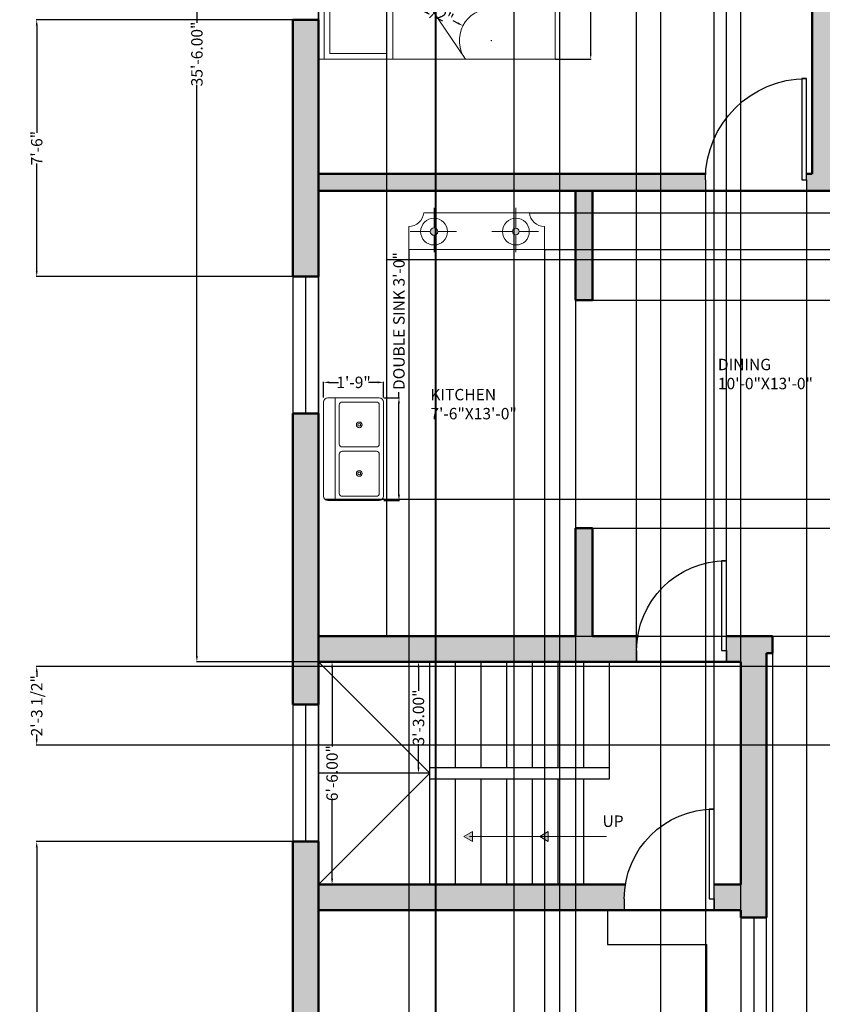
# Model space of a CAD drawing. Units: inches. Extents: x 2430 to 2930, y 1715 to 2575.
# Tile 2 of 4: x 2430 to 2711, y 1933 to 2278. Entities that reach past the tile are written whole.
import ezdxf

# ---------------------------------------------------------------- set-up
doc = ezdxf.new("R2010")
doc.units = ezdxf.units.IN
for name, color, linetype, lineweight in [('A-ANNO-DIMS', 2, 'Continuous', 18), ('A-ANNO-SYMB', 130, 'Continuous', 18), ('A-ANNO-TEXT', 130, 'Continuous', 18), ('A-AREA-IDEN', 130, 'Continuous', 18), ('A-EQPM', 200, 'Continuous', 18), ('A-FLOR', 7, 'Continuous', 25), ('A-FLOR-CASE', 7, 'Continuous', 25), ('A-FLOR-FIXT', 200, 'Continuous', 18), ('A-FLOR-STRS', 7, 'Continuous', 25), ('A-FURN', 200, 'Continuous', 18), ('A-WALL', 7, 'Continuous', 50), ('A-WALL-PATT', 251, 'Continuous', 13), ('DOOR', 224, 'Continuous', 25), ('win', 170, 'Continuous', 25)]:
    doc.layers.add(name, color=color, linetype=linetype, lineweight=lineweight)
doc.styles.get("Standard").update_dxf_attribs({"font": 'arial.ttf', "height": 4})
doc.dimstyles.get("Standard").update_dxf_attribs({"dimtxt": 4, "dimasz": 2, "dimexe": 0.18, "dimexo": 0.0625, "dimgap": 0.09, "dimtad": 0, "dimzin": 0, "dimdsep": 46, "dimlunit": 3, "dimtxsty": 'Standard', "dimcen": 0.09, "dimadec": 0, "dimazin": 0, "dimtfac": 1, "dimtofl": 0, "dimtmove": 0, "dimatfit": 3, "dimfxl": 1, "dimtolj": 1, "dimtzin": 0, "dimarcsym": 0})

# ---------------------------------------------------------------- blocks, each defined once
blk = doc.blocks.new('*D1')
at = {"layer": 'A-ANNO-DIMS', "color": 0, "lineweight": -2, "transparency": 16777216}
for p, q in [((2573.56, 2053.45), (2569.48, 2053.45)), ((2569.66, 2051.45), (2569.66, 2043.24)), ((2569.66, 2016.45), (2569.66, 2024.66)), ((2573.56, 2014.45), (2569.48, 2014.45))]:
    blk.add_line(p, q, dxfattribs=at)
at = {"layer": 'A-ANNO-DIMS', "color": 0, "transparency": 16777216}
for points in [[(2569.32, 2051.45), (2569.99, 2051.45), (2569.66, 2053.45)], [(2569.32, 2016.45), (2569.99, 2016.45), (2569.66, 2014.45)]]:
    blk.add_solid(points, dxfattribs=at)
at = {"layer": 'Defpoints', "color": 0, "transparency": 16777216}
for p in [(2569.66, 2053.45), (2573.62, 2053.45), (2573.62, 2014.45)]:
    blk.add_point(p, dxfattribs=at)
at = {"layer": 'A-ANNO-DIMS', "color": 0, "transparency": 16777216, "insert": (2569.66, 2033.95), "char_height": 4, "attachment_point": 5, "rotation": 90}
blk.add_mtext('\\A1;3\'-3.00"', dxfattribs=at)
blk = doc.blocks.new('*D2')
at = {"layer": 'A-ANNO-DIMS', "color": 0, "lineweight": -2, "transparency": 16777216}
for p, q in [((2534.68, 2053.45), (2539.57, 2053.45)), ((2539.39, 2051.45), (2539.39, 2023.75)), ((2539.39, 1977.45), (2539.39, 2005.15)), ((2534.68, 1975.45), (2539.57, 1975.45))]:
    blk.add_line(p, q, dxfattribs=at)
at = {"layer": 'A-ANNO-DIMS', "color": 0, "transparency": 16777216}
for points in [[(2539.06, 2051.45), (2539.73, 2051.45), (2539.39, 2053.45)], [(2539.06, 1977.45), (2539.73, 1977.45), (2539.39, 1975.45)]]:
    blk.add_solid(points, dxfattribs=at)
at = {"layer": 'Defpoints', "color": 0, "transparency": 16777216}
for p in [(2534.62, 2053.45), (2539.39, 2053.45), (2534.62, 1975.45)]:
    blk.add_point(p, dxfattribs=at)
at = {"layer": 'A-ANNO-DIMS', "color": 0, "transparency": 16777216, "insert": (2539.39, 2014.45), "char_height": 4, "attachment_point": 5, "rotation": 90}
blk.add_mtext('\\A1;6\'-6.00"', dxfattribs=at)
blk = doc.blocks.new('*U5')
for p, q in [((0, 0), (0, -100)), ((800, 0), (800, -100))]:
    blk.add_line(p, q)
blk.add_lwpolyline([(0, 0), (0, 800), (43.75, 800), (43.75, 0)], close=True)
blk.add_arc((0, 0), 800, 0, 90)
blk = doc.blocks.new('*U7')
for p, q in [((0, 0), (0, -100)), ((900, 0), (900, -100))]:
    blk.add_line(p, q)
blk.add_lwpolyline([(0, 0), (0, 900), (43.75, 900), (43.75, 0)], close=True)
blk.add_arc((0, 0), 900, 0, 90)
blk = doc.blocks.new('NEW BED')
for p, q in [((-75.7, 82.92), (0, 82.92)), ((-75.7, 0), (-75.7, 82.92)), ((0, 82.92), (0, 0)), ((-75.7, 80.92), (0, 80.92)), ((-73.7, 78.92), (-39.85, 78.92)), ((-73.7, 58.92), (-73.7, 78.92)), ((-39.85, 58.92), (-39.85, 78.92)), ((-35.85, 78.92), (-2, 78.92)), ((-35.85, 58.92), (-35.85, 78.92)), ((-2, 78.92), (-2, 58.92)), ((-73.7, 58.92), (-39.85, 58.92)), ((-35.85, 58.92), (-2, 58.92)), ((-75.7, 56.92), (0, 56.92)), ((-37.85, 56.92), (-75.7, 31.45)), ((-37.85, 56.92), (-57.85, 22.27)), ((-37.85, 56.92), (0, 31.45)), ((-37.85, 56.92), (-17.84, 22.27)), ((0, 0), (-75.7, 0))]:
    blk.add_line(p, q)
for centre, start, end in [((-69.14, 22.27), 0, 125.5497), ((-6.56, 22.27), 54.4503, 180)]:
    blk.add_arc(centre, 11.28, start, end)
blk = doc.blocks.new('*D13')
at = {"layer": 'A-ANNO-DIMS', "color": 0, "lineweight": -2, "transparency": 16777216}
for p, q in [((2525.56, 2479.45), (2491.85, 2479.45)), ((2492.03, 2477.45), (2492.03, 2277.3)), ((2492.03, 2055.45), (2492.03, 2255.61)), ((2534.56, 2053.45), (2491.85, 2053.45))]:
    blk.add_line(p, q, dxfattribs=at)
at = {"layer": 'A-ANNO-DIMS', "color": 0, "transparency": 16777216}
for points in [[(2491.69, 2477.45), (2492.36, 2477.45), (2492.03, 2479.45)], [(2491.69, 2055.45), (2492.36, 2055.45), (2492.03, 2053.45)]]:
    blk.add_solid(points, dxfattribs=at)
at = {"layer": 'Defpoints', "color": 0, "transparency": 16777216}
for p in [(2525.62, 2479.45), (2492.03, 2053.45), (2534.62, 2053.45)]:
    blk.add_point(p, dxfattribs=at)
at = {"layer": 'A-ANNO-DIMS', "color": 0, "transparency": 16777216, "insert": (2492.03, 2266.45), "char_height": 4, "attachment_point": 5, "rotation": 90}
blk.add_mtext('\\A1;35\'-6.00"', dxfattribs=at)
blk = doc.blocks.new('Sink-double - 36 in top')
for p, q in [((-18, -4), (18, -4)), ((-0.75, -18.5), (-0.75, -6.5)), ((0.75, -6.5), (0.75, -18.5))]:
    blk.add_line(p, q)
for points in [[(-16.5, 0), (16.5, 0)], [(-18, -19.5), (-18, -1.5)], [(18, -1.5), (18, -19.5)], [(-16.5, -18.5), (-16.5, -6.5)], [(-15.5, -5.5), (-1.75, -5.5)], [(1.75, -5.5), (15.5, -5.5)], [(16.5, -6.5), (16.5, -18.5)], [(-1.75, -19.5), (-15.5, -19.5)], [(15.5, -19.5), (1.75, -19.5)], [(16.5, -21), (-16.5, -21)]]:
    blk.add_lwpolyline(points)
for centre, radius in [((-8.5, -12.5), 1), ((-8.5, -12.5), 0.5), ((8.5, -12.5), 1), ((8.5, -12.5), 0.5)]:
    blk.add_circle(centre, radius)
for centre, radius, start, end in [((-16.5, -1.5), 1.5, 90, 180), ((16.5, -1.5), 1.5, 0, 90), ((-15.5, -6.5), 1, 90, 180), ((-1.75, -6.5), 1, 0, 90), ((1.75, -6.5), 1, 90, 180), ((15.5, -6.5), 1, 0, 90), ((-16.5, -19.5), 1.5, 180, 270), ((-15.5, -18.5), 1, 180, 270), ((-1.75, -18.5), 1, 270, 0), ((1.75, -18.5), 1, 180, 270), ((15.5, -18.5), 1, 270, 0), ((16.5, -19.5), 1.5, 270, 0)]:
    blk.add_arc(centre, radius, start, end)
blk = doc.blocks.new('WIN-48IN')
blk.add_line((0, 4.5), (48, 4.5))
blk.add_lwpolyline([(0, 9), (48, 9), (48, 0), (0, 0)], close=True)
blk = doc.blocks.new('*D22')
at = {"layer": 'A-ANNO-DIMS', "color": 0, "lineweight": -2, "transparency": 16777216}
for p, q in [((2617.61, 2340.3), (2630.16, 2340.3)), ((2629.98, 2338.3), (2629.98, 2319.41)), ((2629.98, 2266.6), (2629.98, 2285.5)), ((2617.61, 2264.6), (2630.16, 2264.6))]:
    blk.add_line(p, q, dxfattribs=at)
at = {"layer": 'A-ANNO-DIMS', "color": 0, "transparency": 16777216}
for points in [[(2629.65, 2338.3), (2630.31, 2338.3), (2629.98, 2340.3)], [(2629.65, 2266.6), (2630.31, 2266.6), (2629.98, 2264.6)]]:
    blk.add_solid(points, dxfattribs=at)
at = {"layer": 'Defpoints', "color": 0, "transparency": 16777216}
for p in [(2617.54, 2340.3), (2629.98, 2340.3), (2617.54, 2264.6)]:
    blk.add_point(p, dxfattribs=at)
at = {"layer": 'A-ANNO-DIMS', "color": 0, "transparency": 16777216, "insert": (2629.98, 2302.45), "char_height": 4, "attachment_point": 5, "rotation": 90}
blk.add_mtext('\\A1;6\'-3 1/2" TYP.', dxfattribs=at)
blk = doc.blocks.new('*D23')
at = {"layer": 'A-ANNO-DIMS', "color": 0, "lineweight": -2, "transparency": 16777216}
for p, q in [((2557.48, 2145.98), (2562.99, 2145.98)), ((2562.81, 2145.98), (2562.81, 2147.98)), ((2562.81, 2111.98), (2562.81, 2143.98)), ((2557.48, 2109.98), (2562.99, 2109.98))]:
    blk.add_line(p, q, dxfattribs=at)
at = {"layer": 'A-ANNO-DIMS', "color": 0, "transparency": 16777216}
for points in [[(2562.48, 2143.98), (2563.15, 2143.98), (2562.81, 2145.98)], [(2562.48, 2111.98), (2563.15, 2111.98), (2562.81, 2109.98)]]:
    blk.add_solid(points, dxfattribs=at)
at = {"layer": 'Defpoints', "color": 0, "transparency": 16777216}
for p in [(2557.41, 2145.98), (2562.81, 2145.98), (2557.41, 2109.98)]:
    blk.add_point(p, dxfattribs=at)
at = {"layer": 'A-ANNO-DIMS', "color": 0, "transparency": 16777216, "insert": (2562.81, 2172.85), "char_height": 4, "attachment_point": 5, "rotation": 90}
blk.add_mtext('\\A1;DOUBLE SINK 3\'-0"', dxfattribs=at)
blk = doc.blocks.new('*D24')
at = {"layer": 'A-ANNO-DIMS', "color": 0, "lineweight": -2, "transparency": 16777216}
for p, q in [((2536.41, 2146.05), (2536.41, 2151.56)), ((2538.41, 2151.38), (2541.69, 2151.38)), ((2555.41, 2151.38), (2552.13, 2151.38)), ((2557.41, 2146.05), (2557.41, 2151.56))]:
    blk.add_line(p, q, dxfattribs=at)
at = {"layer": 'A-ANNO-DIMS', "color": 0, "transparency": 16777216}
for points in [[(2538.41, 2151.72), (2538.41, 2151.05), (2536.41, 2151.38)], [(2555.41, 2151.72), (2555.41, 2151.05), (2557.41, 2151.38)]]:
    blk.add_solid(points, dxfattribs=at)
at = {"layer": 'Defpoints', "color": 0, "transparency": 16777216}
for p in [(2536.41, 2151.38), (2536.41, 2145.98), (2557.41, 2145.98)]:
    blk.add_point(p, dxfattribs=at)
at = {"layer": 'A-ANNO-DIMS', "color": 0, "transparency": 16777216, "insert": (2546.91, 2151.38), "char_height": 4, "attachment_point": 5}
blk.add_mtext('\\A1;1\'-9"', dxfattribs=at)
blk = doc.blocks.new('*D26')
at = {"layer": 'A-ANNO-DIMS', "color": 0, "lineweight": -2, "transparency": 16777216}
for p, q in [((2786.56, 2051.85), (2435.74, 2051.85)), ((2435.92, 2049.85), (2435.92, 2048.17)), ((2435.92, 2026.29), (2435.92, 2027.97)), ((2786.56, 2024.29), (2435.74, 2024.29))]:
    blk.add_line(p, q, dxfattribs=at)
at = {"layer": 'A-ANNO-DIMS', "color": 0, "transparency": 16777216}
for points in [[(2435.59, 2049.85), (2436.25, 2049.85), (2435.92, 2051.85)], [(2435.59, 2026.29), (2436.25, 2026.29), (2435.92, 2024.29)]]:
    blk.add_solid(points, dxfattribs=at)
at = {"layer": 'Defpoints', "color": 0, "transparency": 16777216}
for p in [(2435.92, 2051.85), (2786.62, 2051.85), (2786.62, 2024.29)]:
    blk.add_point(p, dxfattribs=at)
at = {"layer": 'A-ANNO-DIMS', "color": 0, "transparency": 16777216, "insert": (2435.92, 2038.07), "char_height": 4, "attachment_point": 5, "rotation": 90}
blk.add_mtext('\\A1;2\'-3 1/2"', dxfattribs=at)
blk = doc.blocks.new('*D30')
at = {"layer": 'A-ANNO-DIMS', "color": 0, "lineweight": -2, "transparency": 16777216}
for p, q in [((2534.62, 2470.39), (2534.62, 1720.57)), ((2575.68, 2470.39), (2575.68, 1720.57)), ((2536.62, 1720.75), (2549.75, 1720.75)), ((2573.68, 1720.75), (2560.56, 1720.75))]:
    blk.add_line(p, q, dxfattribs=at)
at = {"layer": 'A-ANNO-DIMS', "color": 0, "transparency": 16777216}
for points in [[(2536.62, 1721.09), (2536.62, 1720.42), (2534.62, 1720.75)], [(2573.68, 1721.09), (2573.68, 1720.42), (2575.68, 1720.75)]]:
    blk.add_solid(points, dxfattribs=at)
at = {"layer": 'Defpoints', "color": 0, "transparency": 16777216}
for p in [(2534.62, 2470.45), (2575.68, 2470.45), (2575.68, 1720.75)]:
    blk.add_point(p, dxfattribs=at)
at = {"layer": 'A-ANNO-DIMS', "color": 0, "transparency": 16777216, "insert": (2555.15, 1720.75), "char_height": 4, "attachment_point": 5}
blk.add_mtext('\\A1;3\'-5"', dxfattribs=at)
blk = doc.blocks.new('*D33')
at = {"layer": 'A-ANNO-DIMS', "color": 0, "lineweight": -2, "transparency": 16777216}
for p, q in [((2525.56, 2278.45), (2435.74, 2278.45)), ((2435.92, 2276.45), (2435.92, 2238.84)), ((2435.92, 2190.45), (2435.92, 2228.06)), ((2525.56, 2188.45), (2435.74, 2188.45))]:
    blk.add_line(p, q, dxfattribs=at)
at = {"layer": 'A-ANNO-DIMS', "color": 0, "transparency": 16777216}
for points in [[(2435.59, 2276.45), (2436.25, 2276.45), (2435.92, 2278.45)], [(2435.59, 2190.45), (2436.25, 2190.45), (2435.92, 2188.45)]]:
    blk.add_solid(points, dxfattribs=at)
at = {"layer": 'Defpoints', "color": 0, "transparency": 16777216}
for p in [(2525.62, 2278.45), (2435.92, 2188.45), (2525.62, 2188.45)]:
    blk.add_point(p, dxfattribs=at)
at = {"layer": 'A-ANNO-DIMS', "color": 0, "transparency": 16777216, "insert": (2435.92, 2233.45), "char_height": 4, "attachment_point": 5, "rotation": 90}
blk.add_mtext('\\A1;7\'-6"', dxfattribs=at)
blk = doc.blocks.new('*D34')
at = {"layer": 'A-ANNO-DIMS', "color": 0, "lineweight": -2, "transparency": 16777216}
for p, q in [((2525.56, 1990.45), (2435.74, 1990.45)), ((2435.92, 1988.45), (2435.92, 1881.72)), ((2435.92, 1761.45), (2435.92, 1868.18)), ((2525.56, 1759.45), (2435.74, 1759.45))]:
    blk.add_line(p, q, dxfattribs=at)
at = {"layer": 'A-ANNO-DIMS', "color": 0, "transparency": 16777216}
for points in [[(2435.59, 1988.45), (2436.25, 1988.45), (2435.92, 1990.45)], [(2435.59, 1761.45), (2436.25, 1761.45), (2435.92, 1759.45)]]:
    blk.add_solid(points, dxfattribs=at)
at = {"layer": 'Defpoints', "color": 0, "transparency": 16777216}
for p in [(2435.92, 1990.45), (2525.62, 1990.45), (2525.62, 1759.45)]:
    blk.add_point(p, dxfattribs=at)
at = {"layer": 'A-ANNO-DIMS', "color": 0, "transparency": 16777216, "insert": (2435.92, 1874.95), "char_height": 4, "attachment_point": 5, "rotation": 90}
blk.add_mtext('\\A1;19\'-3"', dxfattribs=at)
blk = doc.blocks.new('*D40')
at = {"layer": 'A-ANNO-DIMS', "color": 0, "lineweight": -2, "transparency": 16777216}
for p, q in [((2630.68, 2180.15), (2924.5, 2180.15)), ((2924.32, 2178.15), (2924.32, 2145.66)), ((2924.32, 2102.32), (2924.32, 2134.82)), ((2630.68, 2100.32), (2924.5, 2100.32))]:
    blk.add_line(p, q, dxfattribs=at)
at = {"layer": 'A-ANNO-DIMS', "color": 0, "transparency": 16777216}
for points in [[(2923.99, 2178.15), (2924.65, 2178.15), (2924.32, 2180.15)], [(2923.99, 2102.32), (2924.65, 2102.32), (2924.32, 2100.32)]]:
    blk.add_solid(points, dxfattribs=at)
at = {"layer": 'Defpoints', "color": 0, "transparency": 16777216}
for p in [(2630.62, 2180.15), (2924.32, 2180.15), (2630.62, 2100.32)]:
    blk.add_point(p, dxfattribs=at)
at = {"layer": 'A-ANNO-DIMS', "color": 0, "transparency": 16777216, "insert": (2924.32, 2140.24), "char_height": 4, "attachment_point": 5, "rotation": 90}
blk.add_mtext('\\A1;6\'-8"', dxfattribs=at)
blk = doc.blocks.new('*D41')
at = {"layer": 'A-ANNO-DIMS', "color": 0, "lineweight": -2, "transparency": 16777216}
for p, q in [((2693.62, 2062.39), (2693.62, 1720.57)), ((2750.62, 2056.39), (2750.62, 1720.57)), ((2695.62, 1720.75), (2716.63, 1720.75)), ((2748.62, 1720.75), (2727.61, 1720.75))]:
    blk.add_line(p, q, dxfattribs=at)
at = {"layer": 'A-ANNO-DIMS', "color": 0, "transparency": 16777216}
for points in [[(2695.62, 1721.09), (2695.62, 1720.42), (2693.62, 1720.75)], [(2748.62, 1721.09), (2748.62, 1720.42), (2750.62, 1720.75)]]:
    blk.add_solid(points, dxfattribs=at)
at = {"layer": 'Defpoints', "color": 0, "transparency": 16777216}
for p in [(2693.62, 2062.45), (2750.62, 2056.45), (2750.62, 1720.75)]:
    blk.add_point(p, dxfattribs=at)
at = {"layer": 'A-ANNO-DIMS', "color": 0, "transparency": 16777216, "insert": (2722.12, 1720.75), "char_height": 4, "attachment_point": 5}
blk.add_mtext('\\A1;4\'-9"', dxfattribs=at)
blk = doc.blocks.new('*D42')
at = {"layer": 'A-ANNO-DIMS', "color": 0, "lineweight": -2, "transparency": 16777216}
for p, q in [((2646.07, 2053.52), (2646.07, 2569.33)), ((2648.07, 2569.15), (2651.72, 2569.15)), ((2675.57, 2569.15), (2671.92, 2569.15)), ((2677.57, 2053.52), (2677.57, 2569.33))]:
    blk.add_line(p, q, dxfattribs=at)
at = {"layer": 'A-ANNO-DIMS', "color": 0, "transparency": 16777216}
for points in [[(2648.07, 2569.49), (2648.07, 2568.82), (2646.07, 2569.15)], [(2675.57, 2569.49), (2675.57, 2568.82), (2677.57, 2569.15)]]:
    blk.add_solid(points, dxfattribs=at)
at = {"layer": 'Defpoints', "color": 0, "transparency": 16777216}
for p in [(2677.57, 2569.15), (2646.07, 2053.45), (2677.57, 2053.45)]:
    blk.add_point(p, dxfattribs=at)
at = {"layer": 'A-ANNO-DIMS', "color": 0, "transparency": 16777216, "insert": (2661.82, 2569.15), "char_height": 4, "attachment_point": 5}
blk.add_mtext('\\A1;2\'-7 1/2"', dxfattribs=at)
blk = doc.blocks.new('*D43')
at = {"layer": 'A-ANNO-DIMS', "color": 0, "lineweight": -2, "transparency": 16777216}
for p, q in [((2673.24, 1966.52), (2673.24, 2569.33)), ((2675.24, 2569.15), (2680.62, 2569.15)), ((2682.62, 1966.52), (2682.62, 2569.33)), ((2682.62, 2569.15), (2684.62, 2569.15))]:
    blk.add_line(p, q, dxfattribs=at)
at = {"layer": 'A-ANNO-DIMS', "color": 0, "transparency": 16777216}
for points in [[(2675.24, 2569.49), (2675.24, 2568.82), (2673.24, 2569.15)], [(2680.62, 2569.49), (2680.62, 2568.82), (2682.62, 2569.15)]]:
    blk.add_solid(points, dxfattribs=at)
at = {"layer": 'Defpoints', "color": 0, "transparency": 16777216}
for p in [(2682.62, 2569.15), (2673.24, 1966.45), (2682.62, 1966.45)]:
    blk.add_point(p, dxfattribs=at)
at = {"layer": 'A-ANNO-DIMS', "color": 0, "transparency": 16777216, "insert": (2694.69, 2569.15), "char_height": 4, "attachment_point": 5}
blk.add_mtext('\\A1;0\'-9 1/2"', dxfattribs=at)
blk = doc.blocks.new('*D44')
at = {"layer": 'A-ANNO-DIMS', "color": 0, "lineweight": -2, "transparency": 16777216}
for p, q in [((2670.19, 2218.39), (2670.19, 1720.57)), ((2705.62, 2218.39), (2705.62, 1720.57)), ((2672.19, 1720.75), (2676.25, 1720.75)), ((2703.62, 1720.75), (2699.56, 1720.75))]:
    blk.add_line(p, q, dxfattribs=at)
at = {"layer": 'A-ANNO-DIMS', "color": 0, "transparency": 16777216}
for points in [[(2672.19, 1721.09), (2672.19, 1720.42), (2670.19, 1720.75)], [(2703.62, 1721.09), (2703.62, 1720.42), (2705.62, 1720.75)]]:
    blk.add_solid(points, dxfattribs=at)
at = {"layer": 'Defpoints', "color": 0, "transparency": 16777216}
for p in [(2670.19, 2218.45), (2705.62, 2218.45), (2670.19, 1720.75)]:
    blk.add_point(p, dxfattribs=at)
at = {"layer": 'A-ANNO-DIMS', "color": 0, "transparency": 16777216, "insert": (2687.9, 1720.75), "char_height": 4, "attachment_point": 5}
blk.add_mtext('\\A1;2\'-11 1/2"', dxfattribs=at)
blk = doc.blocks.new('*D45')
at = {"layer": 'A-ANNO-DIMS', "color": 0, "lineweight": -2, "transparency": 16777216}
for p, q in [((2619.01, 2380.39), (2619.01, 1720.57)), ((2654.44, 2380.39), (2654.44, 1720.57)), ((2621.01, 1720.75), (2625.07, 1720.75)), ((2652.44, 1720.75), (2648.38, 1720.75))]:
    blk.add_line(p, q, dxfattribs=at)
at = {"layer": 'A-ANNO-DIMS', "color": 0, "transparency": 16777216}
for points in [[(2621.01, 1721.09), (2621.01, 1720.42), (2619.01, 1720.75)], [(2652.44, 1721.09), (2652.44, 1720.42), (2654.44, 1720.75)]]:
    blk.add_solid(points, dxfattribs=at)
at = {"layer": 'Defpoints', "color": 0, "transparency": 16777216}
for p in [(2619.01, 2380.45), (2654.44, 2380.45), (2654.44, 1720.75)]:
    blk.add_point(p, dxfattribs=at)
at = {"layer": 'A-ANNO-DIMS', "color": 0, "transparency": 16777216, "insert": (2636.72, 1720.75), "char_height": 4, "attachment_point": 5}
blk.add_mtext('\\A1;2\'-11 1/2"', dxfattribs=at)
blk = doc.blocks.new('*D46')
at = {"layer": 'A-ANNO-DIMS', "color": 0, "lineweight": -2, "transparency": 16777216}
for p, q in [((2575.5, 2380.39), (2575.5, 1720.57)), ((2603.06, 2380.39), (2603.06, 1720.57)), ((2577.5, 1720.75), (2579.18, 1720.75)), ((2601.06, 1720.75), (2599.38, 1720.75))]:
    blk.add_line(p, q, dxfattribs=at)
at = {"layer": 'A-ANNO-DIMS', "color": 0, "transparency": 16777216}
for points in [[(2577.5, 1721.09), (2577.5, 1720.42), (2575.5, 1720.75)], [(2601.06, 1721.09), (2601.06, 1720.42), (2603.06, 1720.75)]]:
    blk.add_solid(points, dxfattribs=at)
at = {"layer": 'Defpoints', "color": 0, "transparency": 16777216}
for p in [(2575.5, 2380.45), (2603.06, 2380.45), (2603.06, 1720.75)]:
    blk.add_point(p, dxfattribs=at)
at = {"layer": 'A-ANNO-DIMS', "color": 0, "transparency": 16777216, "insert": (2589.28, 1720.75), "char_height": 4, "attachment_point": 5}
blk.add_mtext('\\A1;2\'-3 1/2"', dxfattribs=at)
blk = doc.blocks.new('*D49')
at = {"layer": 'A-ANNO-DIMS', "color": 0, "lineweight": -2, "transparency": 16777216}
for p, q in [((2534.62, 2062.52), (2534.62, 2569.33)), ((2536.62, 2569.15), (2541.18, 2569.15)), ((2556.62, 2569.15), (2552.06, 2569.15)), ((2558.62, 2062.52), (2558.62, 2569.33))]:
    blk.add_line(p, q, dxfattribs=at)
at = {"layer": 'A-ANNO-DIMS', "color": 0, "transparency": 16777216}
for points in [[(2536.62, 2569.49), (2536.62, 2568.82), (2534.62, 2569.15)], [(2556.62, 2569.49), (2556.62, 2568.82), (2558.62, 2569.15)]]:
    blk.add_solid(points, dxfattribs=at)
at = {"layer": 'Defpoints', "color": 0, "transparency": 16777216}
for p in [(2558.62, 2569.15), (2534.62, 2062.45), (2558.62, 2062.45)]:
    blk.add_point(p, dxfattribs=at)
at = {"layer": 'A-ANNO-DIMS', "color": 0, "transparency": 16777216, "insert": (2546.62, 2569.15), "char_height": 4, "attachment_point": 5}
blk.add_mtext('\\A1;2\'-0"', dxfattribs=at)
blk = doc.blocks.new('*D50')
at = {"layer": 'A-ANNO-DIMS', "color": 0, "lineweight": -2, "transparency": 16777216}
for p, q in [((2536.91, 2110.42), (2924.5, 2110.42)), ((2924.32, 2108.42), (2924.32, 2091.92)), ((2924.32, 2064.45), (2924.32, 2080.95)), ((2534.68, 2062.45), (2924.5, 2062.45))]:
    blk.add_line(p, q, dxfattribs=at)
at = {"layer": 'A-ANNO-DIMS', "color": 0, "transparency": 16777216}
for points in [[(2923.99, 2108.42), (2924.65, 2108.42), (2924.32, 2110.42)], [(2923.99, 2064.45), (2924.65, 2064.45), (2924.32, 2062.45)]]:
    blk.add_solid(points, dxfattribs=at)
at = {"layer": 'Defpoints', "color": 0, "transparency": 16777216}
for p in [(2536.85, 2110.42), (2534.62, 2062.45), (2924.32, 2062.45)]:
    blk.add_point(p, dxfattribs=at)
at = {"layer": 'A-ANNO-DIMS', "color": 0, "transparency": 16777216, "insert": (2924.32, 2086.44), "char_height": 4, "attachment_point": 5, "rotation": 90}
blk.add_mtext('\\A1;4\'-0"', dxfattribs=at)
blk = doc.blocks.new('*D51')
at = {"layer": 'A-ANNO-DIMS', "color": 0, "lineweight": -2, "transparency": 16777216}
for p, q in [((2566.24, 2197.83), (2566.24, 1720.57)), ((2613.75, 2197.83), (2613.75, 1720.57)), ((2568.24, 1720.75), (2578.38, 1720.75)), ((2611.75, 1720.75), (2601.62, 1720.75))]:
    blk.add_line(p, q, dxfattribs=at)
at = {"layer": 'A-ANNO-DIMS', "color": 0, "transparency": 16777216}
for points in [[(2568.24, 1721.09), (2568.24, 1720.42), (2566.24, 1720.75)], [(2611.75, 1721.09), (2611.75, 1720.42), (2613.75, 1720.75)]]:
    blk.add_solid(points, dxfattribs=at)
at = {"layer": 'Defpoints', "color": 0, "transparency": 16777216}
for p in [(2566.24, 2197.89), (2613.75, 2197.89), (2613.75, 1720.75)]:
    blk.add_point(p, dxfattribs=at)
at = {"layer": 'A-ANNO-DIMS', "color": 0, "transparency": 16777216, "insert": (2590, 1720.75), "char_height": 4, "attachment_point": 5}
blk.add_mtext('\\A1;3\'-11 1/2"', dxfattribs=at)
blk = doc.blocks.new('*D52')
at = {"layer": 'A-ANNO-DIMS', "color": 0, "lineweight": -2, "transparency": 16777216}
for p, q in [((2924.32, 2212.78), (2924.32, 2214.78)), ((2608.57, 2210.78), (2924.5, 2210.78)), ((2613.81, 2197.89), (2924.5, 2197.89)), ((2924.32, 2195.89), (2924.32, 2193.89))]:
    blk.add_line(p, q, dxfattribs=at)
at = {"layer": 'A-ANNO-DIMS', "color": 0, "transparency": 16777216}
for points in [[(2923.99, 2212.78), (2924.65, 2212.78), (2924.32, 2210.78)], [(2923.99, 2195.89), (2924.65, 2195.89), (2924.32, 2197.89)]]:
    blk.add_solid(points, dxfattribs=at)
at = {"layer": 'Defpoints', "color": 0, "transparency": 16777216}
for p in [(2608.51, 2210.78), (2924.32, 2210.78), (2613.75, 2197.89)]:
    blk.add_point(p, dxfattribs=at)
at = {"layer": 'A-ANNO-DIMS', "color": 0, "transparency": 16777216, "insert": (2924.32, 2204.34), "char_height": 4, "attachment_point": 5, "rotation": 90}
blk.add_mtext('\\A1;1\'-1"', dxfattribs=at)
blk = doc.blocks.new('*D53')
at = {"layer": 'A-ANNO-DIMS', "color": 0, "lineweight": -2, "transparency": 16777216}
for p, q in [((2613.75, 2197.83), (2613.75, 1720.57)), ((2624.62, 2194.39), (2624.62, 1720.57)), ((2615.75, 1720.75), (2622.62, 1720.75)), ((2624.62, 1720.75), (2626.62, 1720.75))]:
    blk.add_line(p, q, dxfattribs=at)
at = {"layer": 'A-ANNO-DIMS', "color": 0, "transparency": 16777216}
for points in [[(2615.75, 1721.09), (2615.75, 1720.42), (2613.75, 1720.75)], [(2622.62, 1721.09), (2622.62, 1720.42), (2624.62, 1720.75)]]:
    blk.add_solid(points, dxfattribs=at)
at = {"layer": 'Defpoints', "color": 0, "transparency": 16777216}
for p in [(2613.75, 2197.89), (2624.62, 2194.45), (2624.62, 1720.75)]:
    blk.add_point(p, dxfattribs=at)
at = {"layer": 'A-ANNO-DIMS', "color": 0, "transparency": 16777216, "insert": (2633.58, 1720.75), "char_height": 4, "attachment_point": 5}
blk.add_mtext('\\A1;0\'-11"', dxfattribs=at)
blk = doc.blocks.new('*D54')
at = {"layer": 'A-ANNO-DIMS', "color": 0, "lineweight": -2, "transparency": 16777216}
for p, q in [((2624.68, 2218.45), (2924.5, 2218.45)), ((2924.32, 2216.45), (2924.32, 2211.89)), ((2924.32, 2196.45), (2924.32, 2201.01)), ((2624.68, 2194.45), (2924.5, 2194.45))]:
    blk.add_line(p, q, dxfattribs=at)
at = {"layer": 'A-ANNO-DIMS', "color": 0, "transparency": 16777216}
for points in [[(2923.99, 2216.45), (2924.65, 2216.45), (2924.32, 2218.45)], [(2923.99, 2196.45), (2924.65, 2196.45), (2924.32, 2194.45)]]:
    blk.add_solid(points, dxfattribs=at)
at = {"layer": 'Defpoints', "color": 0, "transparency": 16777216}
for p in [(2624.62, 2218.45), (2924.32, 2218.45), (2624.62, 2194.45)]:
    blk.add_point(p, dxfattribs=at)
at = {"layer": 'A-ANNO-DIMS', "color": 0, "transparency": 16777216, "insert": (2924.32, 2206.45), "char_height": 4, "attachment_point": 5, "rotation": 90}
blk.add_mtext('\\A1;2\'-0"', dxfattribs=at)
blk = doc.blocks.new('*D55')
at = {"layer": 'A-ANNO-DIMS', "color": 0, "lineweight": -2, "transparency": 16777216}
for p, q in [((2581.68, 2278.16), (2583.46, 2277.24)), ((2595.18, 2271.16), (2595.36, 2271.16)), ((2595.27, 2271.07), (2595.27, 2271.25))]:
    blk.add_line(p, q, dxfattribs=at)
at = {"layer": 'A-ANNO-DIMS', "color": 0, "transparency": 16777216}
blk.add_solid([(2583.61, 2277.54), (2583.31, 2276.94), (2585.24, 2276.33)], dxfattribs=at)
at = {"layer": 'Defpoints', "color": 0, "transparency": 16777216}
for p in [(2585.24, 2276.33), (2595.27, 2271.16)]:
    blk.add_point(p, dxfattribs=at)
at = {"layer": 'A-ANNO-DIMS', "color": 0, "transparency": 16777216, "insert": (2565.79, 2286.33), "char_height": 4, "attachment_point": 5, "rotation": 332.7752}
blk.add_mtext('\\A1;2X R0\'-11 1/2"', dxfattribs=at)

msp = doc.modelspace()

# ---------------------------------------------------------------- hatches: boundary and pattern name
at = {"layer": 'A-ANNO-SYMB'}
h = msp.add_hatch(color=256, dxfattribs=at)
h.dxf.hatch_style = 1
h.paths.add_polyline_path([(2588.532, 1993.979), (2585.551, 1992.258), (2588.532, 1990.536)])
h.paths.add_polyline_path([(2612.155, 1992.258), (2615.136, 1992.258), (2615.136, 1993.979)])
h.paths.add_polyline_path([(2612.155, 1992.258), (2615.136, 1990.536), (2615.136, 1992.258)])
at = {"layer": 'A-EQPM'}
h = msp.add_hatch(color=256, dxfattribs=at)
h.dxf.hatch_style = 1
h.paths.add_polyline_path([(2602.635, 2204.204, 1), (2604.959, 2204.204, 1)])
h.paths.add_polyline_path([(2576.398, 2204.204, 1), (2573.799, 2204.204, 1)])
at = {"layer": 'A-WALL-PATT'}
h = msp.add_hatch(color=256, dxfattribs=at)
h.dxf.hatch_style = 1
h.paths.add_polyline_path([(2714.621, 2380.453), (2707.621, 2380.453), (2707.621, 2224.453), (2705.621, 2224.453), (2705.621, 2222.39), (2705.621, 2218.453), (2715.188, 2218.453), (2715.188, 2222.39), (2715.188, 2224.453), (2714.621, 2224.453)])
h.paths.add_polyline_path([(2756.969, 2384.39, -0.0145648), (2757.029, 2386.453), (2654.378, 2386.453, -0.0145648), (2654.438, 2384.39), (2654.438, 2380.453), (2756.969, 2380.453)])
h = msp.add_hatch(color=256, dxfattribs=at)
h.dxf.hatch_style = 1
h.paths.add_polyline_path([(2885.621, 2116.453), (2876.621, 2116.453), (2876.621, 2044.453), (2885.621, 2044.453)])
h.paths.add_polyline_path([(2876.621, 2062.453), (2756.621, 2062.453), (2756.621, 2065.333), (2754.558, 2065.333), (2750.621, 2065.333), (2750.621, 2062.453), (2750.621, 2056.453), (2876.621, 2056.453)])
h.paths.add_polyline_path([(2885.621, 2278.453), (2876.621, 2278.453), (2876.621, 2164.453), (2885.621, 2164.453)])
h.paths.add_polyline_path([(2876.621, 2224.453), (2750.561, 2224.453, -0.0145648), (2750.621, 2222.39), (2750.621, 2218.453), (2876.621, 2218.453)])
h.paths.add_polyline_path([(2756.621, 2218.453), (2750.621, 2218.453), (2750.621, 2100.766), (2754.558, 2100.766, -0.0145648), (2756.621, 2100.706)])
h.paths.add_polyline_path([(2630.621, 2100.325), (2624.621, 2100.325), (2624.621, 2062.453), (2534.621, 2062.453), (2534.621, 2053.453), (2646.072, 2053.453), (2646.072, 2057.39, -0.0403846), (2646.482, 2062.453), (2630.621, 2062.453)])
h.paths.add_polyline_path([(2534.621, 2140.453), (2525.621, 2140.453), (2525.621, 2038.453), (2534.621, 2038.453)])
h.paths.add_polyline_path([(2670.188, 2222.39, -0.0145648), (2670.248, 2224.453), (2534.621, 2224.453), (2534.621, 2218.453), (2670.188, 2218.453)])
h.paths.add_polyline_path([(2630.621, 2218.453), (2624.621, 2218.453), (2624.621, 2180.154), (2630.621, 2180.154)])
h.paths.add_polyline_path([(2534.621, 2278.453), (2525.621, 2278.453), (2525.621, 2188.453), (2534.621, 2188.453)])
h = msp.add_hatch(color=256, dxfattribs=at)
h.dxf.hatch_style = 1
h.paths.add_polyline_path([(2885.621, 1897.453), (2876.621, 1897.453), (2876.621, 1769.453), (2682.621, 1769.453), (2682.621, 1759.453), (2885.621, 1759.453)])
h.paths.add_polyline_path([(2885.621, 2020.453), (2876.621, 2020.453), (2876.621, 1945.453), (2885.621, 1945.453)])
h.paths.add_polyline_path([(2876.621, 1840.453), (2808.121, 1840.453), (2808.121, 1831.453), (2876.621, 1831.453)], flags=17)
h.paths.add_polyline_path([(2760.121, 1840.453), (2691.621, 1840.453), (2691.621, 1849.896), (2686.558, 1849.896), (2682.621, 1849.896), (2682.621, 1831.453), (2760.121, 1831.453)], flags=17)
h.paths.add_polyline_path([(2691.621, 1915.889), (2682.621, 1915.889), (2682.621, 1889.266), (2686.558, 1889.266, -0.0322505), (2691.621, 1888.939)])
h.paths.add_polyline_path([(2691.621, 2056.453), (2693.621, 2056.453), (2693.621, 2062.453), (2682.621, 2062.453), (2677.568, 2062.453), (2677.568, 2057.39), (2677.568, 2053.453), (2682.621, 2053.453), (2682.621, 1975.453), (2673.244, 1975.453), (2673.244, 1970.39), (2673.244, 1966.453), (2682.621, 1966.453), (2682.621, 1963.889), (2691.621, 1963.889)])
h.paths.add_polyline_path([(2641.748, 1970.39, -0.0403846), (2642.158, 1975.453), (2534.621, 1975.453), (2534.621, 1966.453), (2641.748, 1966.453)])
h.paths.add_polyline_path([(2534.621, 1990.453), (2525.621, 1990.453), (2525.621, 1759.453), (2534.621, 1759.453)])

# ---------------------------------------------------------------- linework, layer by layer
at = {"layer": 'A-ANNO-SYMB'}
for p, q in [((2635.464, 1992.258), (2587.538, 1992.258)), ((2627.621, 1992.258), (2627.621, 1992.258))]:
    msp.add_line(p, q, dxfattribs=at)
for points in [[(2585.551, 1992.258), (2588.532, 1990.536), (2588.532, 1993.979)], [(2612.155, 1992.258), (2615.136, 1990.536), (2615.136, 1993.979)]]:
    msp.add_lwpolyline(points, close=True, dxfattribs=at)
at = {"layer": 'A-EQPM'}
for p, q in [((2575.098, 2205.504), (2575.098, 2212.561)), ((2603.797, 2205.366), (2603.797, 2212.561)), ((2571.484, 2210.778), (2608.51, 2210.778)), ((2566.245, 2197.895), (2566.245, 2205.997)), ((2613.749, 2205.997), (2613.749, 2197.895)), ((2573.799, 2204.204), (2566.701, 2204.204)), ((2575.098, 2199.512), (2575.098, 2202.904)), ((2579.79, 2204.204), (2576.398, 2204.204)), ((2579.79, 2204.204), (2583, 2204.204)), ((2602.635, 2204.204), (2595.4, 2204.204)), ((2603.797, 2199.512), (2603.797, 2203.042)), ((2608.489, 2204.204), (2604.959, 2204.204)), ((2608.489, 2204.204), (2611.699, 2204.204)), ((2613.749, 2197.895), (2566.245, 2197.895)), ((2575.098, 2199.512), (2575.098, 2197.028)), ((2603.797, 2199.512), (2603.797, 2197.028))]:
    msp.add_line(p, q, dxfattribs=at)
for centre, radius in [((2575.098, 2204.204), 4.692), ((2603.797, 2204.204), 4.692), ((2575.098, 2204.204), 1.3), ((2603.797, 2204.204), 1.162)]:
    msp.add_circle(centre, radius, dxfattribs=at)
for centre, start, end in [((2566.245, 2211.259), 270, 354.7495), ((2613.749, 2211.259), 185.2505, 270)]:
    msp.add_arc(centre, 5.262, start, end, dxfattribs=at)
at = {"layer": 'A-FLOR'}
for p, q in [((2635.872, 1966.453), (2635.872, 1954.453)), ((2635.872, 1954.453), (2670.621, 1954.453)), ((2670.621, 1831.453), (2670.621, 1954.453))]:
    msp.add_line(p, q, dxfattribs=at)
at = {"layer": 'A-FLOR-CASE'}
for p, q in [((2558.621, 2062.453), (2558.621, 2194.453)), ((2558.621, 2194.453), (2624.621, 2194.453))]:
    msp.add_line(p, q, dxfattribs=at)
at = {"layer": 'A-FLOR-STRS'}
for p, q in [((2573.621, 2014.453), (2534.621, 2053.453)), ((2573.621, 1975.453), (2573.621, 2053.453)), ((2582.621, 2016.453), (2582.621, 2053.453)), ((2591.621, 2016.453), (2591.621, 2053.453)), ((2600.621, 2016.453), (2600.621, 2053.453)), ((2609.621, 2016.453), (2609.621, 2053.453)), ((2618.621, 2016.453), (2618.621, 2053.453)), ((2627.621, 2016.453), (2627.621, 2053.453)), ((2636.621, 2012.453), (2636.621, 2053.453)), ((2573.621, 2016.453), (2636.621, 2016.453)), ((2534.621, 1975.453), (2573.621, 2014.453)), ((2573.621, 2014.453), (2534.621, 2014.453)), ((2573.621, 2012.453), (2636.621, 2012.453)), ((2582.621, 1975.453), (2582.621, 2012.453)), ((2591.621, 1975.453), (2591.621, 2012.453)), ((2600.621, 1975.453), (2600.621, 2012.453)), ((2609.621, 1975.453), (2609.621, 2012.453)), ((2618.621, 1975.453), (2618.621, 2012.453)), ((2627.621, 1975.453), (2627.621, 2012.453))]:
    msp.add_line(p, q, dxfattribs=at)
at = {"layer": 'A-WALL'}
for p, q in [((2707.621, 2224.453), (2707.621, 2380.453)), ((2534.621, 2278.453), (2525.621, 2278.453)), ((2534.621, 2188.453), (2534.621, 2278.453)), ((2534.621, 2224.453), (2670.248, 2224.453)), ((2705.621, 2224.453), (2707.621, 2224.453)), ((2534.621, 2218.453), (2876.621, 2218.453)), ((2624.621, 2180.154), (2624.621, 2218.453)), ((2630.621, 2180.154), (2630.621, 2218.453)), ((2534.621, 2188.453), (2525.621, 2188.453)), ((2630.621, 2180.154), (2624.621, 2180.154)), ((2534.621, 2140.453), (2525.621, 2140.453)), ((2534.621, 2038.453), (2534.621, 2140.453)), ((2624.621, 2062.453), (2624.621, 2100.325)), ((2630.621, 2100.325), (2624.621, 2100.325)), ((2630.621, 2062.453), (2630.621, 2100.325)), ((2534.621, 2062.453), (2624.621, 2062.453)), ((2630.621, 2062.453), (2646.482, 2062.453)), ((2677.568, 2062.453), (2682.621, 2062.453)), ((2682.621, 2062.453), (2693.621, 2062.453)), ((2693.621, 2056.453), (2693.621, 2062.453)), ((2691.621, 2056.453), (2693.621, 2056.453)), ((2691.621, 1963.889), (2691.621, 2056.453)), ((2534.621, 2053.453), (2682.621, 2053.453)), ((2682.621, 1975.453), (2682.621, 2053.453)), ((2534.621, 2038.453), (2525.621, 2038.453)), ((2534.621, 1990.453), (2525.621, 1990.453)), ((2534.621, 1759.453), (2534.621, 1990.453)), ((2534.621, 1975.453), (2642.158, 1975.453)), ((2673.244, 1975.453), (2682.621, 1975.453)), ((2534.621, 1966.453), (2682.621, 1966.453)), ((2682.621, 1963.889), (2682.621, 1966.453)), ((2682.621, 1963.889), (2691.621, 1963.889))]:
    msp.add_line(p, q, dxfattribs=at)
for points in [[(2525.621, 2188.453), (2525.621, 2278.453)], [(2525.621, 2038.453), (2525.621, 2140.453)], [(2534.621, 1759.453), (2525.621, 1759.453), (2525.621, 1990.453)]]:
    msp.add_lwpolyline(points, dxfattribs=at)

# ---------------------------------------------------------------- block references
at = {"layer": 'A-FLOR-FIXT', "rotation": 90}
msp.add_blockref('Sink-double - 36 in top', (2536.413, 2127.983), dxfattribs=at)
at = {"layer": 'A-FURN', "rotation": 90}
msp.add_blockref('NEW BED', (2617.543, 2340.302), dxfattribs=at)
at = {"layer": 'DOOR', "xscale": -0.0393700787401575, "yscale": 0.0393700787401575, "zscale": 0.0393700787401575}
for name, p in [('*U7', (2705.621, 2222.39)), ('*U5', (2677.568, 2057.39)), ('*U5', (2673.244, 1970.39))]:
    msp.add_blockref(name, p, dxfattribs=at)
at = {"layer": 'win', "extrusion": (0, 0, -1), "zscale": -1}
for p, rotation in [((-2534.621, 2188.453), 270.0000000000006), ((-2534.621, 2038.453), 270.0000000000005), ((-2691.621, 1963.89), 270.0000000000003)]:
    msp.add_blockref('WIN-48IN', p, dxfattribs=dict(at, rotation=rotation))

# ---------------------------------------------------------------- texts
at = {"layer": 'A-ANNO-TEXT', "insert": (2634.134, 1999.614), "char_height": 4, "attachment_point": 1}
msp.add_mtext_dynamic_manual_height_columns('UP ', width=8.34258, gutter_width=20, heights=[0], dxfattribs=at)
at = {"layer": 'A-AREA-IDEN', "char_height": 4, "attachment_point": 1}
for s, width, insert in [('DINING\\P10\'-0"X13\'-0"', 44.90279, (2674.545, 2159.636)), ('KITCHEN\\P7\'-6"X13\'-0"', 39.46003, (2573.835, 2149.087))]:
    msp.add_mtext_dynamic_manual_height_columns(s, width=width, gutter_width=20, heights=[0], dxfattribs=dict(at, insert=insert))

# ---------------------------------------------------------------- dimensions: what is measured, and where the dimension line sits
at = {"layer": 'A-ANNO-DIMS'}
for base, p1, p2, picture, middle in [((2677.568, 2569.153), (2646.072, 2053.453), (2677.568, 2053.453), '*D42', (2661.82, 2569.153)), ((2682.621, 2569.153), (2673.244, 1966.453), (2682.621, 1966.453), '*D43', (2694.688, 2569.153)), ((2558.621, 2569.153), (2534.621, 2062.453), (2558.621, 2062.453), '*D49', (2546.621, 2569.153)), ((2575.684, 1720.753), (2534.621, 2470.453), (2575.684, 2470.453), '*D30', (2555.153, 1720.753)), ((2603.056, 1720.753), (2575.497, 2380.453), (2603.056, 2380.453), '*D46', (2589.277, 1720.753)), ((2654.438, 1720.753), (2619.005, 2380.453), (2654.438, 2380.453), '*D45', (2636.722, 1720.753)), ((2670.188, 1720.753), (2705.621, 2218.453), (2670.188, 2218.453), '*D44', (2687.905, 1720.753)), ((2613.749, 1720.753), (2566.245, 2197.895), (2613.749, 2197.895), '*D51', (2589.997, 1720.753)), ((2624.621, 1720.753), (2613.749, 2197.895), (2624.621, 2194.453), '*D53', (2633.582, 1720.753)), ((2750.621, 1720.753), (2693.621, 2062.453), (2750.621, 2056.453), '*D41', (2722.121, 1720.753))]:
    dim = msp.add_linear_dim(base=base, p1=p1, p2=p2, dimstyle='Standard', override={"dimdec": 1, "dimlfac": 1, "dimrnd": 0, "dimzin": 1, "dimdsep": 46, "dimlunit": 4, "dimfrac": 2}, dxfattribs=at)
    dim.commit()
    dim.dimension.update_dxf_attribs({"geometry": picture, "text_midpoint": middle})
for base, p1, p2, angle, override, picture, middle in [((2492.026, 2053.453), (2525.621, 2479.453), (2534.621, 2053.453), 90, {"dimclrd": 0, "dimclre": 0, "dimclrt": 0}, '*D13', (2492.026, 2266.453)), ((2435.921, 2188.453), (2525.621, 2278.453), (2525.621, 2188.453), 90, {"dimdec": 1, "dimlfac": 1, "dimrnd": 0, "dimzin": 1, "dimdsep": 46, "dimlunit": 4, "dimfrac": 2}, '*D33', (2435.921, 2233.453)), ((2924.321, 2218.453), (2624.621, 2194.453), (2624.621, 2218.453), 90, {"dimdec": 1, "dimlfac": 1, "dimrnd": 0, "dimzin": 1, "dimdsep": 46, "dimlunit": 4, "dimfrac": 2}, '*D54', (2924.321, 2206.453)), ((2924.321, 2210.778), (2613.749, 2197.895), (2608.51, 2210.778), 90, {"dimdec": 1, "dimlfac": 1, "dimrnd": 0, "dimzin": 1, "dimdsep": 46, "dimlunit": 4, "dimfrac": 2}, '*D52', (2924.321, 2204.336)), ((2924.321, 2180.154), (2630.621, 2100.325), (2630.621, 2180.154), 90, {"dimdec": 1, "dimlfac": 1, "dimrnd": 0, "dimzin": 1, "dimdsep": 46, "dimlunit": 4, "dimfrac": 2}, '*D40', (2924.321, 2140.239)), ((2536.413, 2151.383), (2557.413, 2145.983), (2536.413, 2145.983), 180, {"dimdec": 1, "dimlfac": 1, "dimrnd": 0, "dimzin": 1, "dimdsep": 46, "dimlunit": 4, "dimfrac": 2}, '*D24', (2546.913, 2151.383)), ((2924.321, 2062.453), (2536.852, 2110.422), (2534.621, 2062.453), 90, {"dimdec": 1, "dimlfac": 1, "dimrnd": 0, "dimzin": 1, "dimdsep": 46, "dimlunit": 4, "dimfrac": 2}, '*D50', (2924.321, 2086.438)), ((2539.392, 2053.453), (2534.621, 1975.453), (2534.621, 2053.453), 90, {"dimclrd": 0, "dimclre": 0, "dimclrt": 0}, '*D2', (2539.392, 2014.453)), ((2569.655, 2053.453), (2573.621, 2014.453), (2573.621, 2053.453), 90, {"dimclrd": 0, "dimclre": 0, "dimclrt": 0}, '*D1', (2569.655, 2033.953)), ((2435.921, 2051.847), (2786.621, 2024.288), (2786.621, 2051.847), 90, {"dimdec": 1, "dimlfac": 1, "dimrnd": 0, "dimzin": 1, "dimdsep": 46, "dimlunit": 4, "dimfrac": 2}, '*D26', (2435.921, 2038.067)), ((2435.921, 1990.453), (2525.621, 1759.453), (2525.621, 1990.453), 90, {"dimdec": 1, "dimlfac": 1, "dimrnd": 0, "dimzin": 1, "dimdsep": 46, "dimlunit": 4, "dimfrac": 2}, '*D34', (2435.921, 1874.953))]:
    dim = msp.add_linear_dim(base=base, p1=p1, p2=p2, angle=angle, dimstyle='Standard', override=override, dxfattribs=at)
    dim.commit()
    dim.dimension.update_dxf_attribs({"geometry": picture, "text_midpoint": middle})
for base, p1, p2, text, picture, middle in [((2629.981, 2340.302), (2617.543, 2264.603), (2617.543, 2340.302), '<> TYP.', '*D22', (2629.981, 2302.453)), ((2562.813, 2145.983), (2557.413, 2109.983), (2557.413, 2145.983), 'DOUBLE SINK <>', '*D23', (2562.813, 2172.853))]:
    dim = msp.add_linear_dim(base=base, p1=p1, p2=p2, angle=90, text=text, dimstyle='Standard', override={"dimdec": 1, "dimlfac": 1, "dimrnd": 0, "dimzin": 1, "dimdsep": 46, "dimlunit": 4, "dimfrac": 2}, dxfattribs=at)
    dim.commit()
    dim.dimension.update_dxf_attribs({"geometry": picture, "text_midpoint": middle})
dim = msp.add_radius_dim(center=(2595.271, 2271.164), mpoint=(2585.237, 2276.326), text='2X <>', dimstyle='Standard', override={"dimdec": 1, "dimlfac": 1, "dimrnd": 0, "dimzin": 1, "dimdsep": 46, "dimlunit": 4, "dimfrac": 2}, dxfattribs=at)
dim.commit()
dim.dimension.update_dxf_attribs({"geometry": '*D55', "text_midpoint": (2565.793, 2286.33)})

doc.saveas('drawing.dxf')
